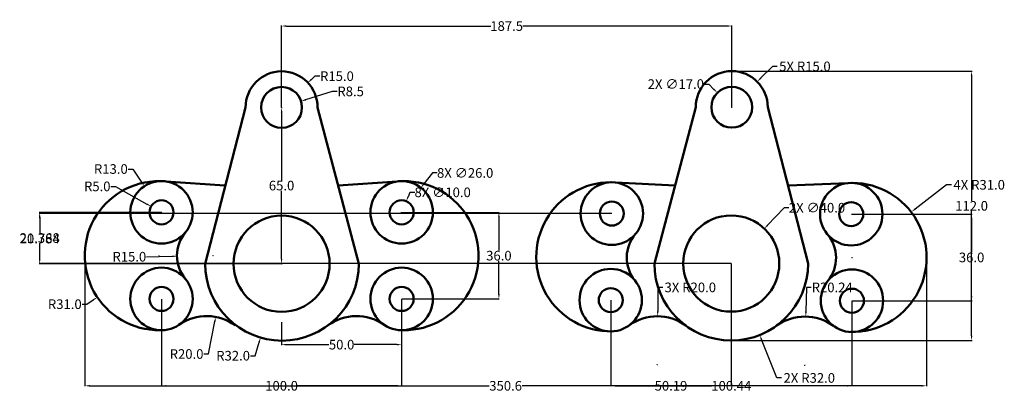
# Model space of a CAD drawing. Units: millimetres. Extents: x 1503 to 1913, y 445 to 600.
import ezdxf

# ---------------------------------------------------------------- set-up
doc = ezdxf.new("R2010")
doc.units = ezdxf.units.MM
doc.header["$MEASUREMENT"] = 0
doc.layers.add('M-DIMS', color=3, linetype='Continuous', lineweight=25)
doc.layers.add('M-OUTL', color=7, linetype='Continuous', lineweight=50)
doc.styles.get("Standard").update_dxf_attribs({"font": 'arial.ttf'})
doc.dimstyles.get("Standard").update_dxf_attribs({"dimtxt": 4, "dimasz": 2, "dimexe": 0.18, "dimexo": 0.0625, "dimgap": 0.09, "dimtad": 0, "dimtih": 1, "dimtoh": 1, "dimdec": 1, "dimzin": 0, "dimdsep": 46, "dimtxsty": 'Standard', "dimcen": 0.09, "dimadec": 0, "dimazin": 0, "dimtfac": 1, "dimtdec": 1, "dimtofl": 0, "dimtmove": 0, "dimatfit": 3, "dimfxl": 1, "dimtolj": 1, "dimtzin": 0, "dimarcsym": 0})

# ---------------------------------------------------------------- blocks, each defined once
blk = doc.blocks.new('*D1')
at = {"layer": 'Defpoints', "color": 0, "transparency": 16777216}
for p in [(1611.88, 563.41), (1611.88, 498.41), (1611.88, 498.41)]:
    blk.add_point(p, dxfattribs=at)
at = {"layer": 'M-DIMS', "color": 0, "lineweight": -2, "transparency": 16777216}
for p, q in [((1611.94, 563.41), (1612.06, 563.41)), ((1611.88, 561.41), (1611.88, 533.04)), ((1611.88, 500.41), (1611.88, 528.77)), ((1611.94, 498.41), (1612.06, 498.41))]:
    blk.add_line(p, q, dxfattribs=at)
at = {"layer": 'M-DIMS', "color": 0, "transparency": 16777216}
for points in [[(1611.55, 561.41), (1612.21, 561.41), (1611.88, 563.41)], [(1611.55, 500.41), (1612.21, 500.41), (1611.88, 498.41)]]:
    blk.add_solid(points, dxfattribs=at)
at = {"layer": 'M-DIMS', "color": 0, "transparency": 16777216, "insert": (1611.88, 530.91), "char_height": 4, "attachment_point": 5}
blk.add_mtext('\\A1;65.0', dxfattribs=at)
blk = doc.blocks.new('*D2')
at = {"layer": 'Defpoints', "color": 0, "transparency": 16777216}
for p in [(1661.88, 519.77), (1702.38, 519.77), (1661.88, 483.77)]:
    blk.add_point(p, dxfattribs=at)
at = {"layer": 'M-DIMS', "color": 0, "lineweight": -2, "transparency": 16777216}
for p, q in [((1661.94, 519.77), (1702.56, 519.77)), ((1702.38, 517.77), (1702.38, 503.91)), ((1702.38, 485.77), (1702.38, 499.64)), ((1661.94, 483.77), (1702.56, 483.77))]:
    blk.add_line(p, q, dxfattribs=at)
at = {"layer": 'M-DIMS', "color": 0, "transparency": 16777216}
for points in [[(1702.05, 517.77), (1702.72, 517.77), (1702.38, 519.77)], [(1702.05, 485.77), (1702.72, 485.77), (1702.38, 483.77)]]:
    blk.add_solid(points, dxfattribs=at)
at = {"layer": 'M-DIMS', "color": 0, "transparency": 16777216, "insert": (1702.38, 501.77), "char_height": 4, "attachment_point": 5}
blk.add_mtext('\\A1;36.0', dxfattribs=at)
blk = doc.blocks.new('*D3')
at = {"layer": 'Defpoints', "color": 0, "transparency": 16777216}
for p in [(1584.44, 476.31), (1580.69, 456.66)]:
    blk.add_point(p, dxfattribs=at)
at = {"layer": 'M-DIMS', "color": 0, "lineweight": -2, "transparency": 16777216}
for p, q in [((1581.5, 460.88), (1584.07, 474.34)), ((1579.5, 460.88), (1581.5, 460.88))]:
    blk.add_line(p, q, dxfattribs=at)
at = {"layer": 'M-DIMS', "color": 0, "transparency": 16777216}
blk.add_solid([(1583.74, 474.41), (1584.4, 474.28), (1584.44, 476.31)], dxfattribs=at)
at = {"layer": 'M-DIMS', "color": 0, "transparency": 16777216, "insert": (1572.31, 460.88), "char_height": 4, "attachment_point": 5}
blk.add_mtext('\\A1;R20.0', dxfattribs=at)
blk = doc.blocks.new('*D4')
at = {"layer": 'Defpoints', "color": 0, "transparency": 16777216}
for p in [(1612.06, 498.41), (1603.09, 467.69)]:
    blk.add_point(p, dxfattribs=at)
at = {"layer": 'M-DIMS', "color": 0, "lineweight": -2, "transparency": 16777216}
for p, q in [((1611.97, 498.41), (1612.15, 498.41)), ((1612.06, 498.32), (1612.06, 498.5)), ((1600.89, 460.16), (1602.53, 465.77)), ((1598.89, 460.16), (1600.89, 460.16))]:
    blk.add_line(p, q, dxfattribs=at)
at = {"layer": 'M-DIMS', "color": 0, "transparency": 16777216}
blk.add_solid([(1602.21, 465.86), (1602.85, 465.68), (1603.09, 467.69)], dxfattribs=at)
at = {"layer": 'M-DIMS', "color": 0, "transparency": 16777216, "insert": (1591.69, 460.16), "char_height": 4, "attachment_point": 5}
blk.add_mtext('\\A1;R32.0', dxfattribs=at)
blk = doc.blocks.new('*D5')
at = {"layer": 'Defpoints', "color": 0, "transparency": 16777216}
for p in [(1568.33, 501.54), (1583.33, 501.77)]:
    blk.add_point(p, dxfattribs=at)
at = {"layer": 'M-DIMS', "color": 0, "lineweight": -2, "transparency": 16777216}
for p, q in [((1555.68, 501.33), (1566.33, 501.5)), ((1583.24, 501.77), (1583.42, 501.77)), ((1583.33, 501.68), (1583.33, 501.86))]:
    blk.add_line(p, q, dxfattribs=at)
at = {"layer": 'M-DIMS', "color": 0, "transparency": 16777216}
blk.add_solid([(1566.32, 501.84), (1566.33, 501.17), (1568.33, 501.54)], dxfattribs=at)
at = {"layer": 'M-DIMS', "color": 0, "transparency": 16777216, "insert": (1548.48, 501.33), "char_height": 4, "attachment_point": 5}
blk.add_mtext('\\A1;R15.0', dxfattribs=at)
blk = doc.blocks.new('*D6')
at = {"layer": 'Defpoints', "color": 0, "transparency": 16777216}
for p in [(1560.88, 501.76), (1535.13, 484.5)]:
    blk.add_point(p, dxfattribs=at)
at = {"layer": 'M-DIMS', "color": 0, "lineweight": -2, "transparency": 16777216}
for p, q in [((1560.79, 501.76), (1560.97, 501.76)), ((1560.88, 501.67), (1560.88, 501.85)), ((1528.79, 481.59), (1530.79, 481.59)), ((1530.79, 481.59), (1533.47, 483.38))]:
    blk.add_line(p, q, dxfattribs=at)
at = {"layer": 'M-DIMS', "color": 0, "transparency": 16777216}
blk.add_solid([(1533.28, 483.66), (1533.65, 483.11), (1535.13, 484.5)], dxfattribs=at)
at = {"layer": 'M-DIMS', "color": 0, "transparency": 16777216, "insert": (1521.6, 481.59), "char_height": 4, "attachment_point": 5}
blk.add_mtext('\\A1;R31.0', dxfattribs=at)
blk = doc.blocks.new('*D7')
at = {"layer": 'Defpoints', "color": 0, "transparency": 16777216}
for p in [(1557.53, 522.23), (1561.88, 519.77)]:
    blk.add_point(p, dxfattribs=at)
at = {"layer": 'M-DIMS', "color": 0, "lineweight": -2, "transparency": 16777216}
for p, q in [((1540.76, 530.57), (1542.76, 530.57)), ((1542.76, 530.57), (1555.78, 523.22)), ((1561.79, 519.77), (1561.97, 519.77)), ((1561.88, 519.68), (1561.88, 519.86))]:
    blk.add_line(p, q, dxfattribs=at)
at = {"layer": 'M-DIMS', "color": 0, "transparency": 16777216}
blk.add_solid([(1555.95, 523.51), (1555.62, 522.93), (1557.53, 522.23)], dxfattribs=at)
at = {"layer": 'M-DIMS', "color": 0, "transparency": 16777216, "insert": (1535.12, 530.57), "char_height": 4, "attachment_point": 5}
blk.add_mtext('\\A1;R5.0', dxfattribs=at)
blk = doc.blocks.new('*D8')
at = {"layer": 'Defpoints', "color": 0, "transparency": 16777216}
for p in [(1554.71, 530.62), (1561.88, 519.77)]:
    blk.add_point(p, dxfattribs=at)
at = {"layer": 'M-DIMS', "color": 0, "lineweight": -2, "transparency": 16777216}
for p, q in [((1547.97, 537.79), (1549.97, 537.79)), ((1549.97, 537.79), (1553.61, 532.29)), ((1561.79, 519.77), (1561.97, 519.77)), ((1561.88, 519.68), (1561.88, 519.86))]:
    blk.add_line(p, q, dxfattribs=at)
at = {"layer": 'M-DIMS', "color": 0, "transparency": 16777216}
blk.add_solid([(1553.89, 532.47), (1553.33, 532.1), (1554.71, 530.62)], dxfattribs=at)
at = {"layer": 'M-DIMS', "color": 0, "transparency": 16777216, "insert": (1540.78, 537.79), "char_height": 4, "attachment_point": 5}
blk.add_mtext('\\A1;R13.0', dxfattribs=at)
blk = doc.blocks.new('*D9')
at = {"layer": 'Defpoints', "color": 0, "transparency": 16777216}
for p in [(1622.83, 573.66), (1611.88, 563.41)]:
    blk.add_point(p, dxfattribs=at)
at = {"layer": 'M-DIMS', "color": 0, "lineweight": -2, "transparency": 16777216}
for p, q in [((1625.75, 576.39), (1624.29, 575.03)), ((1627.75, 576.39), (1625.75, 576.39)), ((1611.79, 563.41), (1611.97, 563.41)), ((1611.88, 563.32), (1611.88, 563.5))]:
    blk.add_line(p, q, dxfattribs=at)
at = {"layer": 'M-DIMS', "color": 0, "transparency": 16777216}
blk.add_solid([(1624.06, 575.27), (1624.52, 574.78), (1622.83, 573.66)], dxfattribs=at)
at = {"layer": 'M-DIMS', "color": 0, "transparency": 16777216, "insert": (1634.94, 576.39), "char_height": 4, "attachment_point": 5}
blk.add_mtext('\\A1;R15.0', dxfattribs=at)
blk = doc.blocks.new('*D10')
at = {"layer": 'Defpoints', "color": 0, "transparency": 16777216}
for p in [(1619.99, 565.96), (1611.88, 563.41)]:
    blk.add_point(p, dxfattribs=at)
at = {"layer": 'M-DIMS', "color": 0, "lineweight": -2, "transparency": 16777216}
for p, q in [((1632.98, 570.06), (1621.89, 566.57)), ((1634.98, 570.06), (1632.98, 570.06)), ((1611.79, 563.41), (1611.97, 563.41)), ((1611.88, 563.32), (1611.88, 563.5))]:
    blk.add_line(p, q, dxfattribs=at)
at = {"layer": 'M-DIMS', "color": 0, "transparency": 16777216}
blk.add_solid([(1621.79, 566.88), (1621.99, 566.25), (1619.99, 565.96)], dxfattribs=at)
at = {"layer": 'M-DIMS', "color": 0, "transparency": 16777216, "insert": (1640.64, 570.06), "char_height": 4, "attachment_point": 5}
blk.add_mtext('\\A1;R8.5', dxfattribs=at)
blk = doc.blocks.new('*D11')
at = {"layer": 'Defpoints', "color": 0, "transparency": 16777216}
for p in [(1661.88, 483.77), (1611.88, 474.23), (1661.88, 464.77)]:
    blk.add_point(p, dxfattribs=at)
at = {"layer": 'M-DIMS', "color": 0, "lineweight": -2, "transparency": 16777216}
for p, q in [((1661.88, 483.71), (1661.88, 464.59)), ((1611.88, 474.16), (1611.88, 464.59)), ((1613.88, 464.77), (1631.6, 464.77)), ((1659.88, 464.77), (1642.16, 464.77))]:
    blk.add_line(p, q, dxfattribs=at)
at = {"layer": 'M-DIMS', "color": 0, "transparency": 16777216}
for points in [[(1613.88, 465.1), (1613.88, 464.43), (1611.88, 464.77)], [(1659.88, 465.1), (1659.88, 464.43), (1661.88, 464.77)]]:
    blk.add_solid(points, dxfattribs=at)
at = {"layer": 'M-DIMS', "color": 0, "transparency": 16777216, "insert": (1636.88, 464.77), "char_height": 4, "attachment_point": 5}
blk.add_mtext('\\A1;50.0', dxfattribs=at)
blk = doc.blocks.new('HOLE-CONCENTRIC-D10-D26')
for radius in [13, 5]:
    blk.add_circle((0, 0), radius)
blk = doc.blocks.new('*D13')
at = {"layer": 'Defpoints', "color": 0, "transparency": 16777216}
for p in [(1799.37, 597.23), (1611.88, 563.41), (1799.37, 563.48)]:
    blk.add_point(p, dxfattribs=at)
at = {"layer": 'M-DIMS', "color": 0, "lineweight": -2, "transparency": 16777216}
for p, q in [((1611.88, 563.47), (1611.88, 597.41)), ((1613.88, 597.23), (1698.96, 597.23)), ((1797.37, 597.23), (1712.29, 597.23)), ((1799.37, 563.54), (1799.37, 597.41))]:
    blk.add_line(p, q, dxfattribs=at)
at = {"layer": 'M-DIMS', "color": 0, "transparency": 16777216}
for points in [[(1613.88, 597.57), (1613.88, 596.9), (1611.88, 597.23)], [(1797.37, 597.57), (1797.37, 596.9), (1799.37, 597.23)]]:
    blk.add_solid(points, dxfattribs=at)
at = {"layer": 'M-DIMS', "color": 0, "transparency": 16777216, "insert": (1705.62, 597.23), "char_height": 4, "attachment_point": 5}
blk.add_mtext('\\A1;187.5', dxfattribs=at)
blk = doc.blocks.new('*D14')
at = {"layer": 'Defpoints', "color": 0, "transparency": 16777216}
for p in [(1561.88, 483.77), (1661.88, 483.77), (1661.88, 447.66)]:
    blk.add_point(p, dxfattribs=at)
at = {"layer": 'M-DIMS', "color": 0, "lineweight": -2, "transparency": 16777216}
for p, q in [((1561.88, 483.71), (1561.88, 447.48)), ((1661.88, 483.71), (1661.88, 447.48)), ((1563.88, 447.66), (1605.24, 447.66)), ((1659.88, 447.66), (1618.52, 447.66))]:
    blk.add_line(p, q, dxfattribs=at)
at = {"layer": 'M-DIMS', "color": 0, "transparency": 16777216}
for points in [[(1563.88, 447.99), (1563.88, 447.32), (1561.88, 447.66)], [(1659.88, 447.99), (1659.88, 447.32), (1661.88, 447.66)]]:
    blk.add_solid(points, dxfattribs=at)
at = {"layer": 'M-DIMS', "color": 0, "transparency": 16777216, "insert": (1611.88, 447.66), "char_height": 4, "attachment_point": 5}
blk.add_mtext('\\A1;100.0', dxfattribs=at)
blk = doc.blocks.new('*D15')
at = {"layer": 'Defpoints', "color": 0, "transparency": 16777216}
for p in [(1561.88, 519.77), (1511.15, 498.41), (1611.88, 498.41)]:
    blk.add_point(p, dxfattribs=at)
at = {"layer": 'M-DIMS', "color": 0, "lineweight": -2, "transparency": 16777216}
for p, q in [((1561.82, 519.77), (1510.97, 519.77)), ((1511.15, 517.77), (1511.15, 511.22)), ((1511.15, 500.41), (1511.15, 506.96)), ((1611.82, 498.41), (1510.97, 498.41))]:
    blk.add_line(p, q, dxfattribs=at)
at = {"layer": 'M-DIMS', "color": 0, "transparency": 16777216}
for points in [[(1510.81, 517.77), (1511.48, 517.77), (1511.15, 519.77)], [(1510.81, 500.41), (1511.48, 500.41), (1511.15, 498.41)]]:
    blk.add_solid(points, dxfattribs=at)
at = {"layer": 'M-DIMS', "color": 0, "transparency": 16777216, "insert": (1511.15, 509.09), "char_height": 4, "attachment_point": 5}
blk.add_mtext('\\A1;21.368', dxfattribs=at)
blk = doc.blocks.new('*D16')
at = {"layer": 'Defpoints', "color": 0, "transparency": 16777216}
for p in [(1748.96, 483.27), (1849.4, 483.02), (1849.4, 447.66)]:
    blk.add_point(p, dxfattribs=at)
at = {"layer": 'M-DIMS', "color": 0, "lineweight": -2, "transparency": 16777216}
for p, q in [((1748.96, 483.2), (1748.96, 447.48)), ((1849.4, 482.96), (1849.4, 447.48)), ((1750.96, 447.66), (1790.98, 447.66)), ((1847.4, 447.66), (1807.37, 447.66))]:
    blk.add_line(p, q, dxfattribs=at)
at = {"layer": 'M-DIMS', "color": 0, "transparency": 16777216}
for points in [[(1750.96, 447.99), (1750.96, 447.32), (1748.96, 447.66)], [(1847.4, 447.99), (1847.4, 447.32), (1849.4, 447.66)]]:
    blk.add_solid(points, dxfattribs=at)
at = {"layer": 'M-DIMS', "color": 0, "transparency": 16777216, "insert": (1799.18, 447.66), "char_height": 4, "attachment_point": 5}
blk.add_mtext('\\A1;100.44', dxfattribs=at)
blk = doc.blocks.new('*D17')
at = {"layer": 'Defpoints', "color": 0, "transparency": 16777216}
for p in [(1849.12, 519.03), (1849.4, 483.02), (1899.24, 483.02)]:
    blk.add_point(p, dxfattribs=at)
at = {"layer": 'M-DIMS', "color": 0, "lineweight": -2, "transparency": 16777216}
for p, q in [((1849.18, 519.03), (1899.42, 519.03)), ((1899.24, 517.03), (1899.24, 503.16)), ((1899.24, 485.02), (1899.24, 498.89)), ((1849.46, 483.02), (1899.42, 483.02))]:
    blk.add_line(p, q, dxfattribs=at)
at = {"layer": 'M-DIMS', "color": 0, "transparency": 16777216}
for points in [[(1898.9, 517.03), (1899.57, 517.03), (1899.24, 519.03)], [(1898.9, 485.02), (1899.57, 485.02), (1899.24, 483.02)]]:
    blk.add_solid(points, dxfattribs=at)
at = {"layer": 'M-DIMS', "color": 0, "transparency": 16777216, "insert": (1899.24, 501.03), "char_height": 4, "attachment_point": 5}
blk.add_mtext('\\A1;36.0', dxfattribs=at)
blk = doc.blocks.new('*D18')
at = {"layer": 'Defpoints', "color": 0, "transparency": 16777216}
for p in [(1799.14, 498.48), (1748.96, 483.27), (1799.14, 447.66)]:
    blk.add_point(p, dxfattribs=at)
at = {"layer": 'M-DIMS', "color": 0, "lineweight": -2, "transparency": 16777216}
for p, q in [((1799.14, 498.42), (1799.14, 447.48)), ((1748.96, 483.2), (1748.96, 447.48)), ((1750.96, 447.66), (1767.21, 447.66)), ((1797.14, 447.66), (1780.89, 447.66))]:
    blk.add_line(p, q, dxfattribs=at)
at = {"layer": 'M-DIMS', "color": 0, "transparency": 16777216}
for points in [[(1750.96, 447.99), (1750.96, 447.32), (1748.96, 447.66)], [(1797.14, 447.99), (1797.14, 447.32), (1799.14, 447.66)]]:
    blk.add_solid(points, dxfattribs=at)
at = {"layer": 'M-DIMS', "color": 0, "transparency": 16777216, "insert": (1774.05, 447.66), "char_height": 4, "attachment_point": 5}
blk.add_mtext('\\A1;50.19', dxfattribs=at)
blk = doc.blocks.new('*D19')
at = {"layer": 'Defpoints', "color": 0, "transparency": 16777216}
for p in [(1511.15, 519.27), (1749.41, 519.27), (1799.14, 498.48)]:
    blk.add_point(p, dxfattribs=at)
at = {"layer": 'M-DIMS', "color": 0, "lineweight": -2, "transparency": 16777216}
for p, q in [((1749.35, 519.27), (1510.97, 519.27)), ((1511.15, 517.27), (1511.15, 511.01)), ((1511.15, 500.48), (1511.15, 506.74)), ((1799.08, 498.48), (1510.97, 498.48))]:
    blk.add_line(p, q, dxfattribs=at)
at = {"layer": 'M-DIMS', "color": 0, "transparency": 16777216}
for points in [[(1510.81, 517.27), (1511.48, 517.27), (1511.15, 519.27)], [(1510.81, 500.48), (1511.48, 500.48), (1511.15, 498.48)]]:
    blk.add_solid(points, dxfattribs=at)
at = {"layer": 'M-DIMS', "color": 0, "transparency": 16777216, "insert": (1511.15, 508.87), "char_height": 4, "attachment_point": 5}
blk.add_mtext('\\A1;20.784', dxfattribs=at)
blk = doc.blocks.new('*D20')
at = {"layer": 'Defpoints', "color": 0, "transparency": 16777216}
for p in [(1799.37, 578.48), (1899.24, 578.48), (1799.14, 466.48)]:
    blk.add_point(p, dxfattribs=at)
at = {"layer": 'M-DIMS', "color": 0, "lineweight": -2, "transparency": 16777216}
for p, q in [((1799.43, 578.48), (1899.42, 578.48)), ((1899.24, 576.48), (1899.24, 524.61)), ((1899.24, 468.48), (1899.24, 520.35)), ((1799.2, 466.48), (1899.42, 466.48))]:
    blk.add_line(p, q, dxfattribs=at)
at = {"layer": 'M-DIMS', "color": 0, "transparency": 16777216}
for points in [[(1898.9, 576.48), (1899.57, 576.48), (1899.24, 578.48)], [(1898.9, 468.48), (1899.57, 468.48), (1899.24, 466.48)]]:
    blk.add_solid(points, dxfattribs=at)
at = {"layer": 'M-DIMS', "color": 0, "transparency": 16777216, "insert": (1899.24, 522.48), "char_height": 4, "attachment_point": 5}
blk.add_mtext('\\A1;112.0', dxfattribs=at)
blk = doc.blocks.new('*D21')
at = {"layer": 'Defpoints', "color": 0, "transparency": 16777216}
for p in [(1529.9, 500.7), (1880.49, 500.63), (1880.49, 447.66)]:
    blk.add_point(p, dxfattribs=at)
at = {"layer": 'M-DIMS', "color": 0, "lineweight": -2, "transparency": 16777216}
for p, q in [((1529.9, 500.63), (1529.9, 447.48)), ((1880.49, 500.57), (1880.49, 447.48)), ((1531.9, 447.66), (1698.36, 447.66)), ((1878.49, 447.66), (1712.03, 447.66))]:
    blk.add_line(p, q, dxfattribs=at)
at = {"layer": 'M-DIMS', "color": 0, "transparency": 16777216}
for points in [[(1531.9, 447.99), (1531.9, 447.32), (1529.9, 447.66)], [(1878.49, 447.99), (1878.49, 447.32), (1880.49, 447.66)]]:
    blk.add_solid(points, dxfattribs=at)
at = {"layer": 'M-DIMS', "color": 0, "transparency": 16777216, "insert": (1705.19, 447.66), "char_height": 4, "attachment_point": 5}
blk.add_mtext('\\A1;350.6', dxfattribs=at)
blk = doc.blocks.new('*D22')
at = {"layer": 'Defpoints', "color": 0, "transparency": 16777216}
for p in [(1809.97, 574.1), (1799.37, 563.48)]:
    blk.add_point(p, dxfattribs=at)
at = {"layer": 'M-DIMS', "color": 0, "lineweight": -2, "transparency": 16777216}
for p, q in [((1816.33, 580.47), (1811.38, 575.51)), ((1818.33, 580.47), (1816.33, 580.47)), ((1799.28, 563.48), (1799.46, 563.48)), ((1799.37, 563.39), (1799.37, 563.57))]:
    blk.add_line(p, q, dxfattribs=at)
at = {"layer": 'M-DIMS', "color": 0, "transparency": 16777216}
blk.add_solid([(1811.14, 575.75), (1811.62, 575.28), (1809.97, 574.1)], dxfattribs=at)
at = {"layer": 'M-DIMS', "color": 0, "transparency": 16777216, "insert": (1829.82, 580.47), "char_height": 4, "attachment_point": 5}
blk.add_mtext('\\A1;5X R15.0', dxfattribs=at)
blk = doc.blocks.new('*D23')
at = {"layer": 'Defpoints', "color": 0, "transparency": 16777216}
for p in [(1768.5, 476.57), (1768.36, 456.57)]:
    blk.add_point(p, dxfattribs=at)
at = {"layer": 'M-DIMS', "color": 0, "lineweight": -2, "transparency": 16777216}
for p, q in [((1768.59, 488.57), (1768.52, 478.57)), ((1770.59, 488.57), (1768.59, 488.57)), ((1768.27, 456.57), (1768.45, 456.57)), ((1768.36, 456.48), (1768.36, 456.66))]:
    blk.add_line(p, q, dxfattribs=at)
at = {"layer": 'M-DIMS', "color": 0, "transparency": 16777216}
blk.add_solid([(1768.19, 478.57), (1768.85, 478.57), (1768.5, 476.57)], dxfattribs=at)
at = {"layer": 'M-DIMS', "color": 0, "transparency": 16777216, "insert": (1782.08, 488.57), "char_height": 4, "attachment_point": 5}
blk.add_mtext('\\A1;3X R20.0', dxfattribs=at)
blk = doc.blocks.new('*D24')
at = {"layer": 'Defpoints', "color": 0, "transparency": 16777216}
for p in [(1830.2, 476.42), (1829.79, 456.18)]:
    blk.add_point(p, dxfattribs=at)
at = {"layer": 'M-DIMS', "color": 0, "lineweight": -2, "transparency": 16777216}
for p, q in [((1830.44, 488.56), (1830.24, 478.42)), ((1832.44, 488.56), (1830.44, 488.56)), ((1829.7, 456.18), (1829.88, 456.18)), ((1829.79, 456.09), (1829.79, 456.27))]:
    blk.add_line(p, q, dxfattribs=at)
at = {"layer": 'M-DIMS', "color": 0, "transparency": 16777216}
blk.add_solid([(1829.9, 478.43), (1830.57, 478.41), (1830.2, 476.42)], dxfattribs=at)
at = {"layer": 'M-DIMS', "color": 0, "transparency": 16777216, "insert": (1841.19, 488.56), "char_height": 4, "attachment_point": 5}
blk.add_mtext('\\A1;R20.24', dxfattribs=at)
blk = doc.blocks.new('*D25')
at = {"layer": 'Defpoints', "color": 0, "transparency": 16777216}
for p in [(1663.79, 524.39), (1659.97, 515.15)]:
    blk.add_point(p, dxfattribs=at)
at = {"layer": 'M-DIMS', "color": 0, "lineweight": -2, "transparency": 16777216}
for p, q in [((1665.32, 528.09), (1664.56, 526.24)), ((1667.32, 528.09), (1665.32, 528.09)), ((1661.79, 519.77), (1661.97, 519.77)), ((1661.88, 519.68), (1661.88, 519.86))]:
    blk.add_line(p, q, dxfattribs=at)
at = {"layer": 'M-DIMS', "color": 0, "transparency": 16777216}
blk.add_solid([(1664.25, 526.37), (1664.86, 526.12), (1663.79, 524.39)], dxfattribs=at)
at = {"layer": 'M-DIMS', "color": 0, "transparency": 16777216, "insert": (1678.97, 528.09), "char_height": 4, "attachment_point": 5}
blk.add_mtext('\\A1;8X ∅10.0', dxfattribs=at)
blk = doc.blocks.new('*D26')
at = {"layer": 'Defpoints', "color": 0, "transparency": 16777216}
for p in [(1669.89, 530.01), (1653.87, 509.54)]:
    blk.add_point(p, dxfattribs=at)
at = {"layer": 'M-DIMS', "color": 0, "lineweight": -2, "transparency": 16777216}
for p, q in [((1674.7, 536.16), (1671.12, 531.59)), ((1676.7, 536.16), (1674.7, 536.16)), ((1661.79, 519.77), (1661.97, 519.77)), ((1661.88, 519.68), (1661.88, 519.86))]:
    blk.add_line(p, q, dxfattribs=at)
at = {"layer": 'M-DIMS', "color": 0, "transparency": 16777216}
blk.add_solid([(1670.86, 531.79), (1671.39, 531.38), (1669.89, 530.01)], dxfattribs=at)
at = {"layer": 'M-DIMS', "color": 0, "transparency": 16777216, "insert": (1688.34, 536.16), "char_height": 4, "attachment_point": 5}
blk.add_mtext('\\A1;8X ∅26.0', dxfattribs=at)
blk = doc.blocks.new('*D27')
at = {"layer": 'Defpoints', "color": 0, "transparency": 16777216}
for p in [(1812.92, 512.99), (1785.37, 483.98)]:
    blk.add_point(p, dxfattribs=at)
at = {"layer": 'M-DIMS', "color": 0, "lineweight": -2, "transparency": 16777216}
for p, q in [((1821.18, 521.69), (1814.29, 514.44)), ((1823.18, 521.69), (1821.18, 521.69)), ((1799.05, 498.48), (1799.23, 498.48)), ((1799.14, 498.39), (1799.14, 498.57))]:
    blk.add_line(p, q, dxfattribs=at)
at = {"layer": 'M-DIMS', "color": 0, "transparency": 16777216}
blk.add_solid([(1814.05, 514.67), (1814.53, 514.21), (1812.92, 512.99)], dxfattribs=at)
at = {"layer": 'M-DIMS', "color": 0, "transparency": 16777216, "insert": (1834.86, 521.69), "char_height": 4, "attachment_point": 5}
blk.add_mtext('\\A1;2X ∅40.0', dxfattribs=at)
blk = doc.blocks.new('*D28')
at = {"layer": 'Defpoints', "color": 0, "transparency": 16777216}
for p in [(1799.14, 498.48), (1811, 468.76)]:
    blk.add_point(p, dxfattribs=at)
at = {"layer": 'M-DIMS', "color": 0, "lineweight": -2, "transparency": 16777216}
for p, q in [((1799.05, 498.48), (1799.23, 498.48)), ((1799.14, 498.39), (1799.14, 498.57)), ((1818.12, 450.93), (1811.74, 466.91)), ((1820.12, 450.93), (1818.12, 450.93))]:
    blk.add_line(p, q, dxfattribs=at)
at = {"layer": 'M-DIMS', "color": 0, "transparency": 16777216}
blk.add_solid([(1812.05, 467.03), (1811.43, 466.78), (1811, 468.76)], dxfattribs=at)
at = {"layer": 'M-DIMS', "color": 0, "transparency": 16777216, "insert": (1831.64, 450.93), "char_height": 4, "attachment_point": 5}
blk.add_mtext('\\A1;2X R32.0', dxfattribs=at)
blk = doc.blocks.new('*D29')
at = {"layer": 'Defpoints', "color": 0, "transparency": 16777216}
for p in [(1874.08, 519.91), (1849.49, 501.03)]:
    blk.add_point(p, dxfattribs=at)
at = {"layer": 'M-DIMS', "color": 0, "lineweight": -2, "transparency": 16777216}
for p, q in [((1888.83, 531.23), (1875.67, 521.12)), ((1890.83, 531.23), (1888.83, 531.23)), ((1849.4, 501.03), (1849.58, 501.03)), ((1849.49, 500.94), (1849.49, 501.12))]:
    blk.add_line(p, q, dxfattribs=at)
at = {"layer": 'M-DIMS', "color": 0, "transparency": 16777216}
blk.add_solid([(1875.46, 521.39), (1875.87, 520.86), (1874.08, 519.91)], dxfattribs=at)
at = {"layer": 'M-DIMS', "color": 0, "transparency": 16777216, "insert": (1902.4, 531.23), "char_height": 4, "attachment_point": 5}
blk.add_mtext('\\A1;4X R31.0', dxfattribs=at)
blk = doc.blocks.new('*D30')
at = {"layer": 'Defpoints', "color": 0, "transparency": 16777216}
for p in [(1793.36, 569.49), (1805.38, 557.47)]:
    blk.add_point(p, dxfattribs=at)
at = {"layer": 'M-DIMS', "color": 0, "lineweight": -2, "transparency": 16777216}
for p, q in [((1787.75, 573.1), (1789.75, 573.1)), ((1789.75, 573.1), (1791.94, 570.91)), ((1799.28, 563.48), (1799.46, 563.48)), ((1799.37, 563.39), (1799.37, 563.57))]:
    blk.add_line(p, q, dxfattribs=at)
at = {"layer": 'M-DIMS', "color": 0, "transparency": 16777216}
blk.add_solid([(1792.18, 571.14), (1791.71, 570.67), (1793.36, 569.49)], dxfattribs=at)
at = {"layer": 'M-DIMS', "color": 0, "transparency": 16777216, "insert": (1776.07, 573.1), "char_height": 4, "attachment_point": 5}
blk.add_mtext('\\A1;2X ∅17.0', dxfattribs=at)

msp = doc.modelspace()

# ---------------------------------------------------------------- linework, layer by layer
at = {"layer": 'M-OUTL'}
for p, q in [((1596.8799, 563.4068), (1580.0599, 498.4068)), ((1626.8799, 563.4068), (1644.0599, 498.4068)), ((1784.3685, 563.4824), (1767.1355, 498.4824)), ((1814.3685, 563.4824), (1831.1355, 498.4824)), ((1563.7094, 532.6451), (1588.2899, 530.9068)), ((1660.0503, 532.6451), (1635.4699, 530.9068)), ((1748.9488, 532.2713), (1749.1232, 532.2629)), ((1750.9406, 532.1756), (1775.752, 530.9824)), ((1847.6455, 531.9432), (1822.8286, 530.8694)), ((1849.6377, 532.0294), (1849.4633, 532.0219))]:
    msp.add_line(p, q, dxfattribs=at)
for centre, radius in [((1611.8799, 563.4068), 8.5), ((1799.3685, 563.4824), 8.5), ((1611.8799, 498.4068), 20), ((1799.145, 498.4824), 20)]:
    msp.add_circle(centre, radius, dxfattribs=at)
for centre, radius, start, end in [((1611.8799, 563.4068), 15, 360, 180), ((1799.3685, 563.4824), 15, 0, 180), ((1560.8799, 501.7584), 31, 89.408198, 274.516782), ((1662.8799, 501.7584), 31, 265.483218, 90.591802), ((1748.9488, 501.2713), 31, 90, 270.916701), ((1849.4888, 501.0298), 31, 268.808013, 89.724714), ((1583.3275, 501.7745), 15, 139.994799, 220.005201), ((1770.627, 500.9959), 15, 139.269237, 219.28727), ((1827.8095, 500.8586), 15, 320.437444, 40.455477), ((1612.0599, 498.4068), 32, 180, 0), ((1799.1355, 498.4824), 32, 180, 360), ((1580.6932, 456.6625), 20, 53.395921, 124.757273), ((1643.0665, 456.6625), 20, 55.242727, 126.604079), ((1768.3555, 456.5708), 20, 53.706375, 126.006576), ((1829.7892, 456.1847), 20.2386, 53.938463, 125.443188)]:
    msp.add_arc(centre, radius, start, end, dxfattribs=at)

# ---------------------------------------------------------------- block references
for p in [(1561.8799, 519.7745), (1661.8799, 519.7745), (1749.409, 519.2661), (1849.115, 519.0266), (1561.8799, 483.7745), (1661.8799, 483.7745), (1748.9555, 483.2661), (1849.3956, 483.0248)]:
    msp.add_blockref('HOLE-CONCENTRIC-D10-D26', p, dxfattribs=at)

# ---------------------------------------------------------------- dimensions: what is measured, and where the dimension line sits
at = {"layer": 'M-DIMS'}
for base, p1, p2, override, picture, middle in [((1799.3685, 597.2324), (1611.8799, 563.4068), (1799.3685, 563.4824), {"dimdec": 1, "dimlfac": 1, "dimrnd": 0, "dimzin": 0, "dimdsep": 46, "dimlunit": 2}, '*D13', (1705.6242, 597.2324)), ((1880.4862, 447.6568), (1529.898, 500.6968), (1880.4862, 500.6329), {"dimdec": 1, "dimlfac": 1, "dimrnd": 0, "dimzin": 0, "dimdsep": 46, "dimlunit": 2}, '*D21', (1705.1921, 447.6568)), ((1799.145, 447.6568), (1748.9555, 483.2661), (1799.145, 498.4824), {"dimdec": 2, "dimlfac": 1, "dimrnd": 0, "dimzin": 0, "dimdsep": 46, "dimlunit": 2}, '*D18', (1774.0503, 447.6568)), ((1661.8799, 447.6568), (1561.8799, 483.7745), (1661.8799, 483.7745), {"dimdec": 1, "dimlfac": 1, "dimrnd": 0, "dimzin": 0, "dimdsep": 46, "dimlunit": 2}, '*D14', (1611.8799, 447.6568)), ((1661.8799, 464.7667), (1611.8799, 474.226), (1661.8799, 483.7745), {"dimclrd": 0, "dimclre": 0, "dimclrt": 0}, '*D11', (1636.8799, 464.7667)), ((1849.3956, 447.6568), (1748.9555, 483.2661), (1849.3956, 483.0248), {"dimdec": 2, "dimlfac": 1, "dimrnd": 0, "dimzin": 0, "dimdsep": 46, "dimlunit": 2}, '*D16', (1799.1755, 447.6568))]:
    dim = msp.add_linear_dim(base=base, p1=p1, p2=p2, dimstyle='Standard', override=override, dxfattribs=at)
    dim.commit()
    dim.dimension.update_dxf_attribs({"geometry": picture, "text_midpoint": middle})
for center, mpoint, text, picture, middle in [((1799.3685, 563.4824), (1809.9671, 574.0971), '5X <>', '*D22', (1829.816, 580.4658)), ((1849.4888, 501.0298), (1874.0786, 519.9068), '4X <>', '*D29', (1902.4027, 531.233)), ((1799.1355, 498.4824), (1810.9989, 468.7628), '2X <>', '*D28', (1831.6408, 450.9309)), ((1768.3555, 456.5708), (1768.5046, 476.5702), '3X <>', '*D23', (1782.0825, 488.5699))]:
    dim = msp.add_radius_dim(center=center, mpoint=mpoint, text=text, dimstyle='Standard', override={"dimdec": 1, "dimlfac": 1, "dimrnd": 0, "dimzin": 0, "dimdsep": 46, "dimlunit": 2}, dxfattribs=at)
    dim.commit()
    dim.dimension.update_dxf_attribs({"geometry": picture, "text_midpoint": middle, "dimtype": 164})
dim = msp.add_radius_dim(center=(1611.8799, 563.4068), mpoint=(1622.8284, 573.6601), dimstyle='Standard', override={"dimclrd": 0, "dimclre": 0, "dimclrt": 0}, dxfattribs=at)
dim.commit()
dim.dimension.update_dxf_attribs({"geometry": '*D9', "text_midpoint": (1634.9404, 576.3943)})
for p1, p2, text, picture, middle in [((1805.3794, 557.4725), (1793.3576, 569.4924), '2X <>', '*D30', (1776.0717, 573.0983)), ((1653.8693, 509.5358), (1669.8904, 530.0132), '8X <>', '*D26', (1688.3446, 536.1565)), ((1659.9678, 515.1545), (1663.7919, 524.3945), '8X <>', '*D25', (1678.9694, 528.0905)), ((1785.3743, 483.9784), (1812.9157, 512.9865), '2X <>', '*D27', (1834.8575, 521.689))]:
    dim = msp.add_diameter_dim_2p(p1=p1, p2=p2, text=text, dimstyle='Standard', override={"dimdec": 1, "dimlfac": 1, "dimrnd": 0, "dimzin": 0, "dimdsep": 46, "dimlunit": 2}, dxfattribs=at)
    dim.commit()
    dim.dimension.update_dxf_attribs({"geometry": picture, "text_midpoint": middle, "dimtype": 163})
for base, p1, p2, override, picture, middle in [((1899.2362, 578.4824), (1799.1355, 466.4824), (1799.3685, 578.4824), {"dimdec": 1, "dimlfac": 1, "dimrnd": 0, "dimzin": 0, "dimdsep": 46, "dimlunit": 2}, '*D20', (1899.2362, 522.4824)), ((1611.8799, 498.4068), (1611.8799, 563.4068), (1611.8799, 498.4068), {"dimclrd": 0, "dimclre": 0, "dimclrt": 0}, '*D1', (1611.8799, 530.9068)), ((1511.148, 498.4068), (1561.8799, 519.7745), (1611.8799, 498.4068), {"dimdec": 3, "dimlfac": 1, "dimrnd": 0, "dimzin": 0, "dimdsep": 46, "dimlunit": 2}, '*D15', (1511.148, 509.0907)), ((1511.148, 519.2661), (1799.145, 498.4824), (1749.409, 519.2661), {"dimdec": 3, "dimlfac": 1, "dimrnd": 0, "dimzin": 0, "dimdsep": 46, "dimlunit": 2}, '*D19', (1511.148, 508.8743)), ((1899.2362, 483.0248), (1849.115, 519.0266), (1849.3956, 483.0248), {"dimdec": 1, "dimlfac": 1, "dimrnd": 0, "dimzin": 0, "dimdsep": 46, "dimlunit": 2}, '*D17', (1899.2362, 501.0257))]:
    dim = msp.add_linear_dim(base=base, p1=p1, p2=p2, angle=90, dimstyle='Standard', override=override, dxfattribs=at)
    dim.commit()
    dim.dimension.update_dxf_attribs({"geometry": picture, "text_midpoint": middle})
for center, mpoint, override, picture, middle in [((1611.8799, 563.4068), (1619.986, 565.9642), {"dimclrd": 0, "dimclre": 0, "dimclrt": 0}, '*D10', (1640.6367, 570.0625)), ((1561.8799, 519.7745), (1554.7117, 530.6197), {"dimclrd": 0, "dimclre": 0, "dimclrt": 0}, '*D8', (1540.782, 537.7871)), ((1561.8799, 519.7745), (1557.5259, 522.2327), {"dimclrd": 0, "dimclre": 0, "dimclrt": 0}, '*D7', (1535.1194, 530.5706)), ((1560.8799, 501.7584), (1535.1294, 484.4981), {"dimclrd": 0, "dimclre": 0, "dimclrt": 0}, '*D6', (1521.5968, 481.5888)), ((1583.3275, 501.7745), (1568.3294, 501.5353), {"dimclrd": 0, "dimclre": 0, "dimclrt": 0}, '*D5', (1555.6764, 501.3334)), ((1612.0599, 498.4068), (1603.0861, 467.6909), {"dimclrd": 0, "dimclre": 0, "dimclrt": 0}, '*D4', (1591.6936, 460.1597)), ((1829.7892, 456.1847), (1830.1964, 476.4192), {"dimdec": 2, "dimlfac": 1, "dimrnd": 0, "dimzin": 0, "dimdsep": 46, "dimlunit": 2}, '*D24', (1841.1855, 488.5599)), ((1580.6932, 456.6625), (1584.443, 476.3079), {"dimclrd": 0, "dimclre": 0, "dimclrt": 0}, '*D3', (1572.3052, 460.8763))]:
    dim = msp.add_radius_dim(center=center, mpoint=mpoint, dimstyle='Standard', override=override, dxfattribs=at)
    dim.commit()
    dim.dimension.update_dxf_attribs({"geometry": picture, "text_midpoint": middle, "dimtype": 164})
dim = msp.add_linear_dim(base=(1702.3847, 519.7745), p1=(1661.8799, 483.7745), p2=(1661.8799, 519.7745), angle=90, dimstyle='Standard', override={"dimclrd": 0, "dimclre": 0, "dimclrt": 0}, dxfattribs=at)
dim.commit()
dim.dimension.update_dxf_attribs({"geometry": '*D2', "text_midpoint": (1702.3847, 501.7745), "dimtype": 160})

doc.saveas('drawing.dxf')
